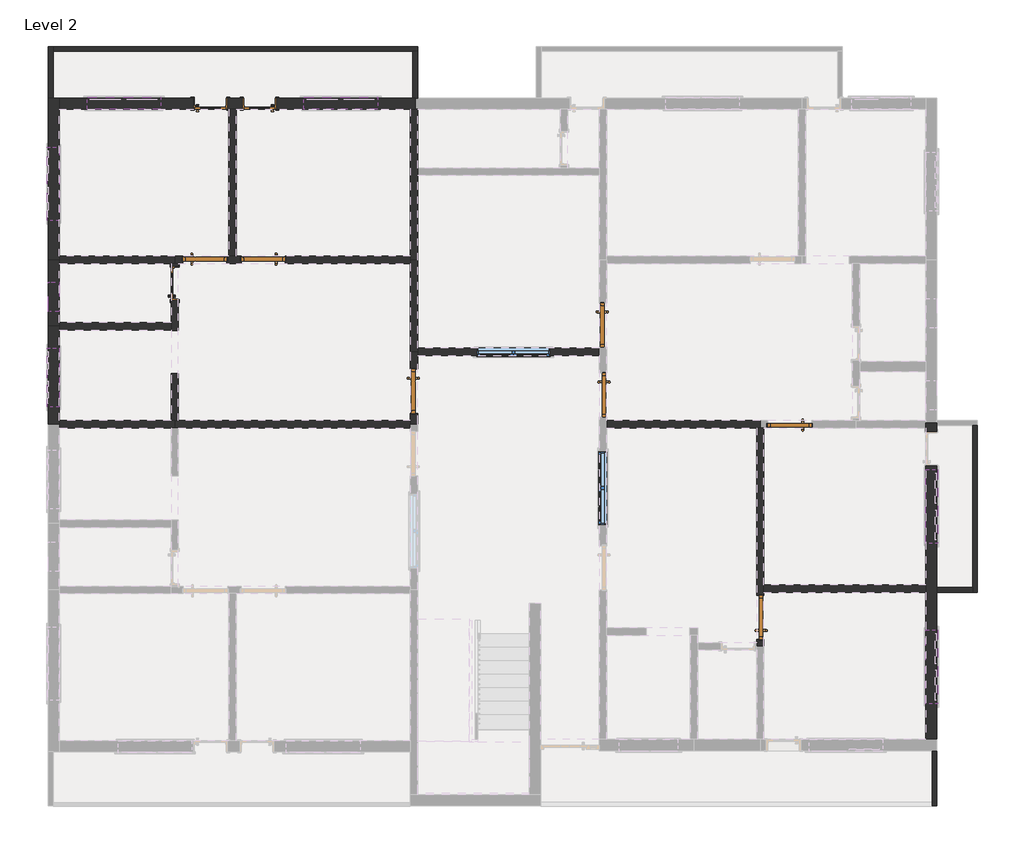
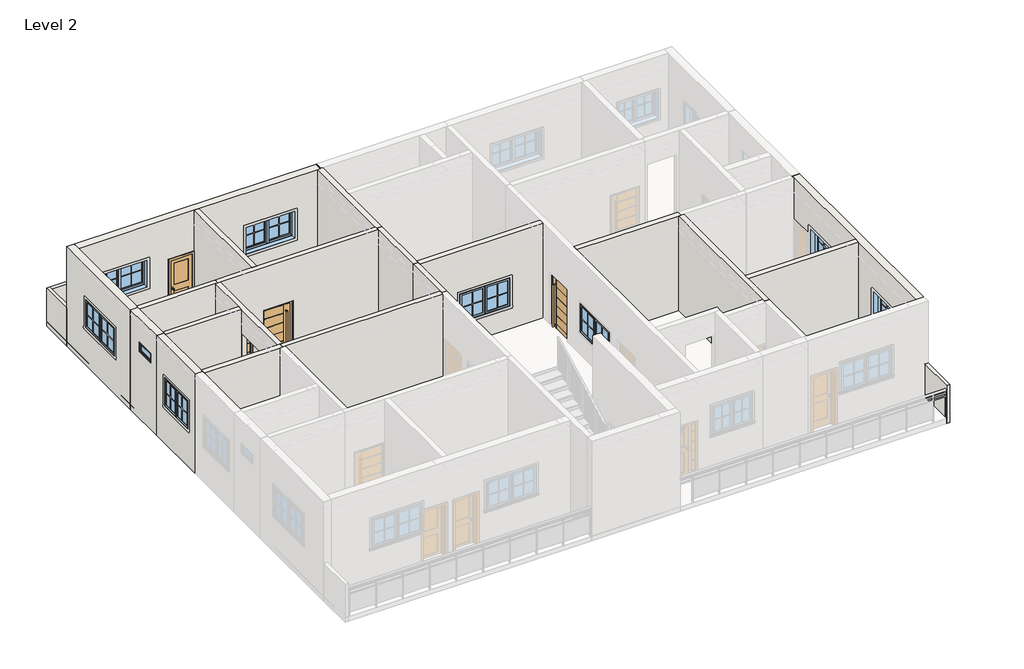
# One storey, part 2 of 5: 25 walls, 10 doors, 9 windows.
# Revit data of these elements (continued)
# Element 42 (IfcWindow, "M_Window-Awning-Double-Horizontal : 5'")
#   Mark = "32"
#   Window Inset = 0' - 0"
#   Interior Wall Closure = 0' - 2 5/32"
#   Frame Extension = 0' - 0 1/4"
#   Exterior Wall Closure = 0' - 1 1/4"
#   Interior Trim Visibility = yes
#   Exterior Trim Visibility = yes
#   Phase Created = New Construction
#   Materials on its faces: "Wood - Stained", "Glass", "Clad - White"
# Element 43 (IfcWindow, "M_Window-Awning-Double-Horizontal : 5'")
#   Mark = "38"
#   Window Inset = 0' - 0"
#   Interior Wall Closure = 0' - 2.15551"
#   Frame Extension = 0' - 0 1/4"
#   Exterior Wall Closure = 0' - 1 1/4"
#   Interior Trim Visibility = yes
#   Exterior Trim Visibility = yes
#   Phase Created = New Construction
#   Materials on its faces: "Wood - Stained", "Glass", "Clad - White"
# Element 44 (IfcWindow, "M_Window-Awning-Double-Horizontal : 5'")
#   Mark = "40"
#   Window Inset = 0' - 0"
#   Interior Wall Closure = 0' - 2.15551"
#   Frame Extension = 0' - 0 1/4"
#   Exterior Wall Closure = 0' - 1 1/4"
#   Interior Trim Visibility = yes
#   Exterior Trim Visibility = yes
#   Phase Created = New Construction
#   Materials on its faces: "Wood - Stained", "Glass", "Clad - White"
# Materials
#   "Cherry": class "Wood", colour RGB 226 177 128, transparency 0, Description = "Prunus Serotina", Cost = 0
#   "Aluminum": class "Metal", colour RGB 247 247 247, transparency 0, Description = "Aluminum 6061", Cost = 0
#   "Glass": class "Glass", colour RGB 0 128 192, transparency 0.75, Description = "Soda Lime Glass", Cost = 0
#   "Sash": class "Wood", colour RGB 224 178 126, transparency 0, Cost = 0
#   "Wood - Stained": class "Wood", colour RGB 224 178 126, transparency 0, Cost = 0
#   "Clad - White": class "Wood", colour RGB 242 242 238, transparency 0, Cost = 0
#   "Default Wall": colour RGB 128 128 128, transparency 0, Cost = 0
#   "OW1": class "Generic", colour RGB 120 120 120, transparency 0, Cost = 0
#   "BRW2": class "Generic", colour RGB 120 120 120, transparency 0, Cost = 0
#   "BW1": class "Generic", colour RGB 120 120 120, transparency 0, Cost = 0
#   "BRW1": class "Generic", colour RGB 120 120 120, transparency 0, Cost = 0
#   "KW2": class "Generic", colour RGB 120 120 120, transparency 0, Cost = 0
#   "KW1": class "Generic", colour RGB 120 120 120, transparency 0, Cost = 0
#   "LVW1": class "Generic", colour RGB 120 120 120, transparency 0, Cost = 0
#   "LVW2": class "Generic", colour RGB 120 120 120, transparency 0, Cost = 0
#   "BRW4": class "Generic", colour RGB 120 120 120, transparency 0, Cost = 0
#   "BRW3": class "Generic", colour RGB 120 120 120, transparency 0, Cost = 0
